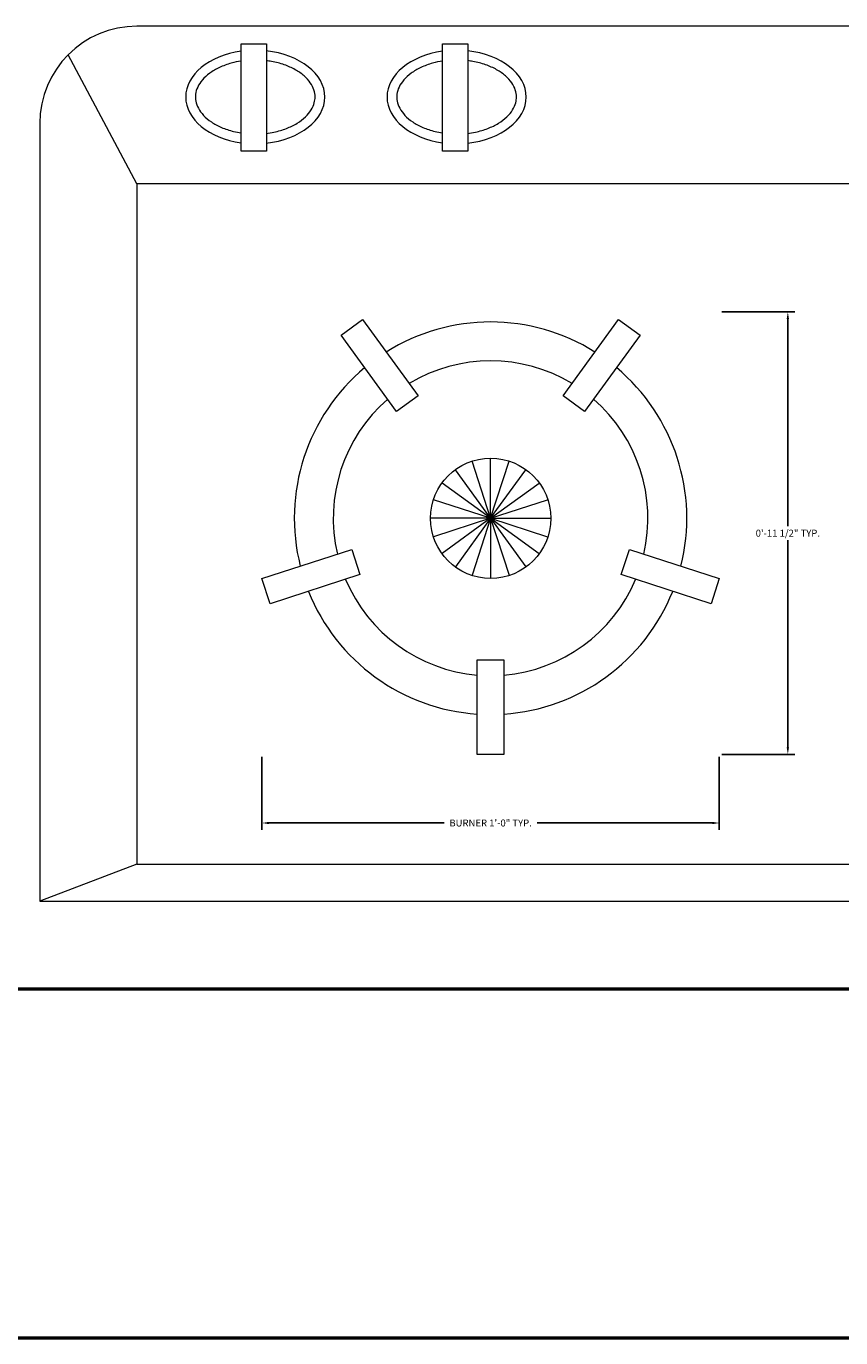
# Model space of a CAD drawing. Units: inches. Extents: x -173 to 545, y -746 to 104.
# Tile 4 of 32: x 182 to 203, y -697 to -664. Entities that reach past the tile are written whole.
import ezdxf

# ---------------------------------------------------------------- set-up
doc = ezdxf.new("R2010")
doc.units = ezdxf.units.IN
doc.header["$MEASUREMENT"] = 0
for name, color, linetype, lineweight in [('A-ANNO-DIMS', 2, 'Continuous', 18), ('A-EQPM', 8, 'Continuous', 18), ('A-WALL', 7, 'Continuous', 50)]:
    doc.layers.add(name, color=color, linetype=linetype, lineweight=lineweight)
doc.styles.get("Standard").update_dxf_attribs({"font": 'arial.ttf'})
doc.dimstyles.get("Standard").update_dxf_attribs({"dimtxt": 0.18, "dimasz": 0.18, "dimexe": 0.18, "dimexo": 0.0625, "dimgap": 0.09, "dimtad": 0, "dimtih": 1, "dimtoh": 1, "dimdec": 0, "dimzin": 0, "dimdsep": 46, "dimlunit": 3, "dimtxsty": 'Standard', "dimcen": 0.09, "dimadec": 0, "dimazin": 0, "dimtfac": 1, "dimtdec": 0, "dimtofl": 0, "dimtmove": 0, "dimatfit": 3, "dimfxl": 1, "dimtolj": 1, "dimtzin": 0, "dimarcsym": 0})

# ---------------------------------------------------------------- blocks, each defined once
blk = doc.blocks.new('HOB-40-BURNER')
for p, q in [((2.04, 10.813), (2.594, 11.215)), ((2.594, 11.215), (4.025, 9.246)), ((7.767, 9.246), (9.198, 11.215)), ((9.198, 11.215), (9.752, 10.813)), ((3.471, 8.844), (2.04, 10.813)), ((9.752, 10.813), (8.321, 8.844)), ((4.025, 9.246), (3.471, 8.844)), ((8.321, 8.844), (7.767, 9.246)), ((5.896, 6.088), (5.419, 7.557)), ((5.896, 6.088), (5.896, 7.633)), ((5.896, 6.088), (6.373, 7.557)), ((5.896, 6.088), (4.988, 7.338)), ((5.896, 6.088), (6.804, 7.338)), ((5.896, 6.088), (4.647, 6.996)), ((5.896, 6.088), (7.145, 6.996)), ((5.896, 6.088), (4.428, 6.566)), ((5.896, 6.088), (7.365, 6.566)), ((5.896, 6.088), (4.352, 6.088)), ((5.896, 6.088), (4.428, 5.611)), ((5.896, 6.088), (4.647, 5.181)), ((5.896, 6.088), (4.988, 4.839)), ((5.896, 6.088), (5.419, 4.62)), ((5.896, 6.088), (7.44, 6.088)), ((5.896, 6.088), (7.365, 5.611)), ((5.896, 6.088), (7.145, 5.181)), ((5.896, 6.088), (6.804, 4.839)), ((5.896, 6.088), (6.373, 4.62)), ((5.896, 6.088), (5.896, 4.544)), ((0, 4.532), (2.315, 5.285)), ((2.315, 5.285), (2.527, 4.634)), ((9.266, 4.634), (9.477, 5.285)), ((9.477, 5.285), (11.792, 4.532)), ((0.211, 3.882), (0, 4.532)), ((2.527, 4.634), (0.211, 3.882)), ((11.581, 3.882), (9.266, 4.634)), ((11.792, 4.532), (11.581, 3.882)), ((5.554, 2.434), (6.238, 2.434)), ((5.554, 0), (5.554, 2.434)), ((6.238, 2.434), (6.238, 0)), ((6.238, 0), (5.554, 0))]:
    blk.add_line(p, q)
blk.add_circle((5.896, 6.088), 1.551)
for radius, start, end in [(5.061, 57.8765, 122.1235), (4.058, 58.8365, 121.1635), (5.061, 129.8765, 194.1235), (5.061, 345.8765, 50.1235), (4.058, 130.8365, 193.1635), (4.058, 346.8365, 49.1635), (4.058, 202.8365, 265.1635), (4.058, 274.8365, 337.1635), (5.061, 201.8765, 266.1235), (5.061, 273.8765, 338.1235)]:
    blk.add_arc((5.896, 6.088), radius, start, end)
blk = doc.blocks.new('*D68')
at = {"layer": 'A-ANNO-DIMS', "color": 0, "lineweight": -2, "transparency": 16777216}
for p, q in [((187.583, -682.383), (187.583, -684.269)), ((199.375, -682.383), (199.375, -684.269)), ((187.763, -684.089), (192.279, -684.089)), ((199.195, -684.089), (194.679, -684.089))]:
    blk.add_line(p, q, dxfattribs=at)
at = {"layer": 'A-ANNO-DIMS', "color": 0, "transparency": 16777216}
for points in [[(187.763, -684.059), (187.763, -684.119), (187.583, -684.089)], [(199.195, -684.059), (199.195, -684.119), (199.375, -684.089)]]:
    blk.add_solid(points, dxfattribs=at)
at = {"layer": 'Defpoints', "color": 0, "transparency": 16777216}
for p in [(187.583, -682.32), (199.375, -682.32), (199.375, -684.089)]:
    blk.add_point(p, dxfattribs=at)
at = {"layer": 'A-ANNO-DIMS', "color": 0, "transparency": 16777216, "insert": (193.479, -684.089), "char_height": 0.18, "attachment_point": 5}
blk.add_mtext('\\A1;BURNER 1\'-0" TYP.', dxfattribs=at)
blk = doc.blocks.new('*D69')
at = {"layer": 'A-ANNO-DIMS', "color": 0, "lineweight": -2, "transparency": 16777216}
for p, q in [((199.438, -670.913), (201.324, -670.913)), ((201.144, -671.093), (201.144, -676.433)), ((201.144, -682.14), (201.144, -676.8)), ((199.438, -682.32), (201.324, -682.32))]:
    blk.add_line(p, q, dxfattribs=at)
at = {"layer": 'A-ANNO-DIMS', "color": 0, "transparency": 16777216}
for points in [[(201.114, -671.093), (201.174, -671.093), (201.144, -670.913)], [(201.114, -682.14), (201.174, -682.14), (201.144, -682.32)]]:
    blk.add_solid(points, dxfattribs=at)
at = {"layer": 'Defpoints', "color": 0, "transparency": 16777216}
for p in [(199.375, -670.913), (201.144, -670.913), (199.375, -682.32)]:
    blk.add_point(p, dxfattribs=at)
at = {"layer": 'A-ANNO-DIMS', "color": 0, "transparency": 16777216, "insert": (201.144, -676.616), "char_height": 0.18, "attachment_point": 5}
blk.add_mtext('\\A1;0\'-11 1/2" TYP.', dxfattribs=at)

msp = doc.modelspace()

# ---------------------------------------------------------------- linework, layer by layer
at = {"layer": 'A-EQPM'}
for p, q in [((219.455, -663.545), (184.36, -663.545)), ((187.047, -666.77), (187.047, -663.997)), ((187.047, -663.997), (187.696, -663.997)), ((187.696, -663.997), (187.696, -666.77)), ((192.24, -666.77), (192.24, -663.997)), ((192.24, -663.997), (192.889, -663.997)), ((192.889, -663.997), (192.889, -666.77)), ((184.36, -667.606), (182.588, -664.279)), ((181.854, -666.052), (181.854, -686.106)), ((187.696, -666.77), (187.047, -666.77)), ((192.889, -666.77), (192.24, -666.77)), ((184.36, -667.606), (184.36, -685.154)), ((219.455, -667.606), (184.36, -667.606)), ((184.36, -685.154), (181.854, -686.106)), ((184.36, -685.154), (219.455, -685.154)), ((181.854, -686.106), (221.961, -686.106))]:
    msp.add_line(p, q, dxfattribs=at)
msp.add_arc((184.36, -666.052), 2.507, 90, 180, dxfattribs=at)
for centre, major_axis, start_param, end_param in [((187.41, -665.37), (1.794, 0), 1.774361, 4.508825), ((187.41, -665.37), (-1.794, 0), 1.73081, 4.552375), ((192.603, -665.37), (1.794, 0), 1.774361, 4.508825), ((192.603, -665.37), (-1.794, 0), 1.73081, 4.552375)]:
    msp.add_ellipse(centre, major_axis=major_axis, ratio=0.671641, start_param=start_param, end_param=end_param, dxfattribs=at)
for points, knots in [([(187.047, -664.443), (186.96, -664.457), (186.874, -664.475), (186.684, -664.528), (186.582, -664.565), (186.395, -664.653), (186.31, -664.703), (186.162, -664.812), (186.099, -664.87), (185.995, -664.99), (185.955, -665.052), (185.897, -665.175), (185.879, -665.236), (185.863, -665.357), (185.865, -665.417), (185.888, -665.539), (185.91, -665.6), (185.976, -665.723), (186.021, -665.784), (186.133, -665.903), (186.2, -665.96), (186.357, -666.066), (186.445, -666.114), (186.638, -666.197), (186.742, -666.231), (186.916, -666.274), (186.981, -666.287), (187.047, -666.297)], [8.079302, 8.079302, 8.079302, 8.079302, 8.245651, 8.245651, 8.463703, 8.463703, 8.681755, 8.681755, 8.899807, 8.899807, 9.117859, 9.117859, 9.33591, 9.33591, 9.553962, 9.553962, 9.772014, 9.772014, 9.990066, 9.990066, 10.208118, 10.208118, 10.426169, 10.426169, 10.644221, 10.644221, 10.770253, 10.770253, 10.770253, 10.770253]), ([(187.696, -666.308), (187.763, -666.3), (187.829, -666.289), (188.005, -666.252), (188.113, -666.22), (188.312, -666.143), (188.405, -666.098), (188.57, -665.997), (188.642, -665.941), (188.765, -665.825), (188.814, -665.764), (188.891, -665.641), (188.917, -665.58), (188.947, -665.469), (188.953, -665.42), (188.953, -665.37), (188.953, -665.31), (188.944, -665.249), (188.903, -665.127), (188.873, -665.065), (188.788, -664.943), (188.734, -664.883), (188.603, -664.768), (188.527, -664.714), (188.355, -664.617), (188.259, -664.574), (188.054, -664.502), (187.944, -664.474), (187.786, -664.445), (187.741, -664.438), (187.696, -664.433)], [4.889299, 4.889299, 4.889299, 4.889299, 5.015191, 5.015191, 5.233243, 5.233243, 5.451295, 5.451295, 5.669347, 5.669347, 5.887399, 5.887399, 6.10545, 6.10545, 6.283185, 6.283185, 6.283185, 6.501237, 6.501237, 6.719289, 6.719289, 6.937341, 6.937341, 7.155392, 7.155392, 7.373444, 7.373444, 7.591496, 7.591496, 7.677072, 7.677072, 7.677072, 7.677072]), ([(192.24, -664.443), (192.153, -664.457), (192.067, -664.475), (191.877, -664.528), (191.775, -664.565), (191.589, -664.653), (191.504, -664.703), (191.355, -664.812), (191.292, -664.87), (191.188, -664.99), (191.148, -665.052), (191.09, -665.175), (191.072, -665.236), (191.056, -665.357), (191.058, -665.417), (191.082, -665.539), (191.103, -665.6), (191.17, -665.723), (191.214, -665.784), (191.326, -665.903), (191.394, -665.96), (191.55, -666.066), (191.638, -666.114), (191.831, -666.197), (191.936, -666.231), (192.109, -666.274), (192.174, -666.287), (192.24, -666.297)], [8.079302, 8.079302, 8.079302, 8.079302, 8.245651, 8.245651, 8.463703, 8.463703, 8.681755, 8.681755, 8.899807, 8.899807, 9.117859, 9.117859, 9.33591, 9.33591, 9.553962, 9.553962, 9.772014, 9.772014, 9.990066, 9.990066, 10.208118, 10.208118, 10.426169, 10.426169, 10.644221, 10.644221, 10.770253, 10.770253, 10.770253, 10.770253]), ([(192.889, -666.308), (192.956, -666.3), (193.022, -666.289), (193.199, -666.252), (193.306, -666.22), (193.506, -666.143), (193.598, -666.098), (193.763, -665.997), (193.836, -665.941), (193.958, -665.825), (194.008, -665.764), (194.084, -665.641), (194.111, -665.58), (194.14, -665.469), (194.147, -665.42), (194.147, -665.37), (194.147, -665.31), (194.137, -665.249), (194.097, -665.127), (194.066, -665.065), (193.981, -664.943), (193.927, -664.883), (193.797, -664.768), (193.72, -664.714), (193.548, -664.617), (193.452, -664.574), (193.247, -664.502), (193.138, -664.474), (192.98, -664.445), (192.934, -664.438), (192.889, -664.433)], [4.889299, 4.889299, 4.889299, 4.889299, 5.015191, 5.015191, 5.233243, 5.233243, 5.451295, 5.451295, 5.669347, 5.669347, 5.887399, 5.887399, 6.10545, 6.10545, 6.283185, 6.283185, 6.283185, 6.501237, 6.501237, 6.719289, 6.719289, 6.937341, 6.937341, 7.155392, 7.155392, 7.373444, 7.373444, 7.591496, 7.591496, 7.677072, 7.677072, 7.677072, 7.677072])]:
    msp.add_open_spline(points, degree=3, knots=knots, dxfattribs=at)
at = {"layer": 'A-WALL'}
for p, q in [((169.801, -688.362), (260.801, -688.362)), ((24.301, -697.362), (501.801, -697.362))]:
    msp.add_line(p, q, dxfattribs=at)

# ---------------------------------------------------------------- block references
at = {"layer": 'A-EQPM'}
msp.add_blockref('HOB-40-BURNER', (187.583, -682.32), dxfattribs=at)

# ---------------------------------------------------------------- dimensions: what is measured, and where the dimension line sits
at = {"layer": 'A-ANNO-DIMS'}
dim = msp.add_linear_dim(base=(201.144, -670.913), p1=(199.375, -682.32), p2=(199.375, -670.913), angle=90, text='<> TYP.', dimstyle='Standard', override={"dimdec": 1, "dimlfac": 1, "dimrnd": 0, "dimzin": 1, "dimdsep": 46, "dimlunit": 4, "dimfrac": 2}, dxfattribs=at)
dim.commit()
dim.dimension.update_dxf_attribs({"geometry": '*D69', "text_midpoint": (201.144, -676.616)})
dim = msp.add_linear_dim(base=(199.375, -684.089), p1=(187.583, -682.32), p2=(199.375, -682.32), text='BURNER <> TYP.', dimstyle='Standard', override={"dimdec": 1, "dimlfac": 1, "dimrnd": 0, "dimzin": 1, "dimdsep": 46, "dimlunit": 4, "dimfrac": 2}, dxfattribs=at)
dim.commit()
dim.dimension.update_dxf_attribs({"geometry": '*D68', "text_midpoint": (193.479, -684.089)})

doc.saveas('drawing.dxf')
